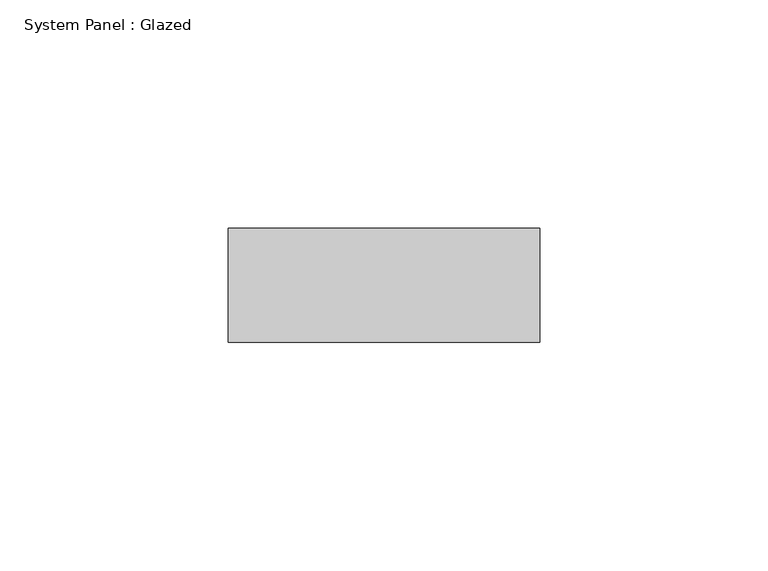
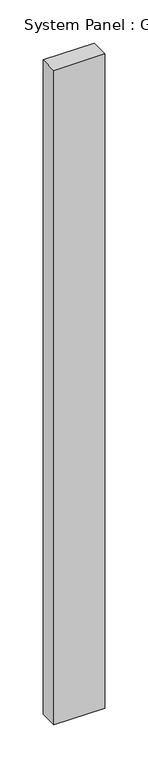
"""IFC4 building model written with IfcOpenShell, lengths in millimetres: plate geometry, System Panel : Glazed."""

from ifc_helpers import new_model, si_unit, origin, origin_with_axes, place, context, project, spatial, polyline, outline, extrude, source, transform, mapped, element, save


def system_panel_glazed_f67349ae(model_context):
    return source(origin(), model_context, "Body", "SweptSolid", [
        extrude(outline(polyline([(34.2076443, 24.5), (-34.2076443, 24.5), (-34.2076443, 49.5), (34.2076443, 49.5), (34.2076443, 24.5)])), origin_with_axes(), (0.0, 0.0, 1.0), 927.5595785),
    ])


if __name__ == "__main__":
    model = new_model("IFC4")
    model_context = context("Model", 3, world=origin())
    ifc_project = project(units=[si_unit("LENGTHUNIT", "METRE", prefix="MILLI")], contexts=[model_context])
    site = spatial("IfcSite", under=ifc_project)
    building = spatial("IfcBuilding", under=site)
    placement = place(None, origin())
    system_panel_glazed_shape = system_panel_glazed_f67349ae(model_context)
    element("IfcPlate", 1, ObjectType="System Panel : Glazed", at=placement, inside=building, context=model_context, shape_type="MappedRepresentation", body=[
        mapped(system_panel_glazed_shape, transform((0.0, 0.0, 0.0), x_axis=(1.0, 0.0, 0.0), y_axis=(0.0, 1.0, 0.0), z_axis=(0.0, 0.0, 1.0))),
    ])
    save(model, "model.ifc")

# Revit data of these elements
# Type "System Panel : Glazed"
#   Construction Type Id = "GSP4R"
#   Analytic Construction = "1/8 in Pilkington single glazing"
#   Visual Light Transmittance = 0.9
#   Solar Heat Gain Coefficient = 0.86
#   Heat Transfer Coefficient (U) = 6.7069 W/(m²·K)
# Element 1 (IfcPlate, "System Panel : Glazed")
#   Materials on its faces: "Glass"
# Materials
#   "Glass": class "Glass", colour RGB 0 128 192, transparency 0.9, Description = "Soda Lime Glass", Cost = 0
